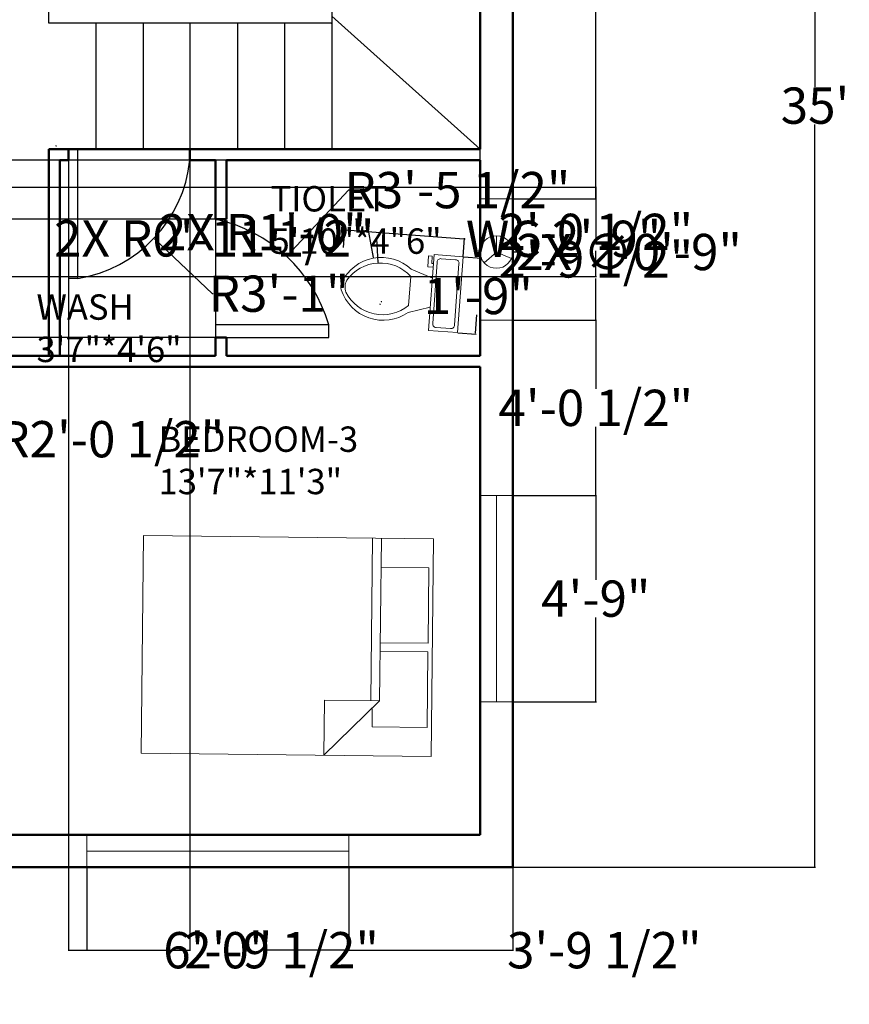
# Model space of a CAD drawing. Units: inches. Extents: x 430 to 924, y 262 to 758.
# Tile 2 of 3: x 695 to 924, y 262 to 534. Entities that reach past the tile are written whole.
import ezdxf

# ---------------------------------------------------------------- set-up
doc = ezdxf.new("R2010")
doc.units = ezdxf.units.IN
doc.header["$MEASUREMENT"] = 0
for name, color, linetype, lineweight in [('A-ANNO-DIMS', 2, 'Continuous', 18), ('A-AREA-IDEN', 7, 'Continuous', 25), ('A-DOOR', 4, 'Continuous', 25), ('A-FLOR-FIXT', 9, 'Continuous', 18), ('A-FLOR-STRS', 7, 'Continuous', 25), ('A-FURN', 9, 'Continuous', 18), ('A-GLAZ', 3, 'Continuous', 18), ('A-WALL', 7, 'Continuous', 50), ('M-HVAC-EQPM', 4, 'Continuous', 18)]:
    doc.layers.add(name, color=color, linetype=linetype, lineweight=lineweight)
doc.styles.get("Standard").update_dxf_attribs({"font": 'arial.ttf'})
doc.dimstyles.get("Standard").update_dxf_attribs({"dimtxt": 10, "dimasz": 0.18, "dimexe": 0.18, "dimexo": 0.0625, "dimgap": 0.09, "dimtad": 0, "dimtih": 1, "dimtoh": 1, "dimdec": 0, "dimzin": 0, "dimdsep": 46, "dimlunit": 3, "dimtxsty": 'Standard', "dimcen": 0.09, "dimadec": 0, "dimazin": 0, "dimtfac": 1, "dimtdec": 0, "dimtofl": 0, "dimtmove": 0, "dimatfit": 3, "dimfxl": 1, "dimtolj": 1, "dimtzin": 0, "dimarcsym": 0})

# ---------------------------------------------------------------- blocks, each defined once
blk = doc.blocks.new('Bed - Queen')
for p, q in [((0, -80.00003), (0, 0)), ((0, 0), (59.99999, 0)), ((59.99999, 0), (59.99999, -80.00003)), ((7.99999, -1.2), (28.79998, -1.2)), ((7.99999, -14.4), (7.99999, -1.2)), ((28.79998, -1.2), (28.79998, -14.4)), ((31.19999, -1.2), (51.99999, -1.2)), ((31.19999, -14.4), (31.19999, -1.2)), ((51.99999, -1.2), (51.99999, -16.4)), ((0, -14.4), (44.8, -14.4)), ((59.99999, -29.6), (44.8, -14.4)), ((44.8, -14.4), (44.8, -29.6)), ((44.8, -16.8), (0, -16.8)), ((51.99999, -16.4), (46.79936, -16.4)), ((44.8, -29.6), (59.99999, -29.6)), ((59.99999, -80.00003), (0, -80.00003))]:
    blk.add_line(p, q)
blk = doc.blocks.new('Toilet - top')
for p, q in [((9.5, -6), (9.5, -2)), ((-8, -8.5), (-8, -8)), ((-7, -8), (-7, -9.5)), ((-4, -8), (-6, -14)), ((4, -8), (6, -14)), ((-10, -8.5), (-8, -8.5)), ((-10, -9.5), (-10, -8.5)), ((-7, -9.5), (-10, -9.5)), ((4, -14), (-4, -14))]:
    blk.add_line(p, q)
blk.add_lwpolyline([(10.5, -8), (10.5, 0), (-10.5, 0), (-10.5, -8)], close=True)
for points in [[(-9.5, -2), (-9.5, -6)], [(8.5, -1), (-8.5, -1)], [(-8.5, -7), (8.5, -7)]]:
    blk.add_lwpolyline(points)
for centre, radius, start, end in [((-8.62, -1.88), 0.884, 81.8699, 188.1301), ((8.62, -1.88), 0.884, 351.8699, 98.1301), ((-8.62, -6.12), 0.884, 171.8699, 278.1301), ((8.62, -6.12), 0.884, 261.8699, 8.1301), ((3.52, -21.58), 12.17, 141.4691, 247.9714), ((4.2, -21.82), 11.33, 136.3677, 238.9468), ((-3.52, -21.58), 12.17, 292.0284, 38.5307), ((-4.2, -21.82), 11.33, 301.053, 43.6321), ((0, -27.88), 4, 245.7318, 294.2682), ((0, -29), 4, 254.8605, 285.1395)]:
    blk.add_arc(centre, radius, start, end)
blk = doc.blocks.new('*D6')
at = {"layer": 'A-ANNO-DIMS', "color": 0, "lineweight": -2, "transparency": 16777216}
for p, q in [((831.38, 720.05), (914.81, 720.05)), ((914.63, 719.87), (914.63, 515.25)), ((914.63, 300.23), (914.63, 504.86)), ((831.38, 300.05), (914.81, 300.05))]:
    blk.add_line(p, q, dxfattribs=at)
at = {"layer": 'A-ANNO-DIMS', "color": 0, "transparency": 16777216}
for points in [[(914.6, 719.87), (914.66, 719.87), (914.63, 720.05)], [(914.6, 300.23), (914.66, 300.23), (914.63, 300.05)]]:
    blk.add_solid(points, dxfattribs=at)
at = {"layer": 'Defpoints', "color": 0, "transparency": 16777216}
for p in [(831.32, 720.05), (831.32, 300.05), (914.63, 300.05)]:
    blk.add_point(p, dxfattribs=at)
at = {"layer": 'A-ANNO-DIMS', "color": 0, "transparency": 16777216, "insert": (914.63, 510.05), "char_height": 10, "attachment_point": 5}
blk.add_mtext("\\A1;35'", dxfattribs=at)
blk = doc.blocks.new('*D13')
at = {"layer": 'A-ANNO-DIMS', "color": 0, "lineweight": -2, "transparency": 16777216}
for p, q in [((784.63, 470.89), (785, 475.95)), ((785.17, 475.76), (817.77, 473.36)), ((817.59, 468.46), (817.96, 473.52)), ((817.95, 473.34), (818.13, 473.33))]:
    blk.add_line(p, q, dxfattribs=at)
at = {"layer": 'A-ANNO-DIMS', "color": 0, "transparency": 16777216}
for points in [[(785.17, 475.79), (785.17, 475.73), (784.99, 475.77)], [(817.77, 473.39), (817.77, 473.33), (817.95, 473.34)]]:
    blk.add_solid(points, dxfattribs=at)
at = {"layer": 'Defpoints', "color": 0, "transparency": 16777216}
for p in [(817.95, 473.34), (784.63, 470.83), (817.58, 468.4)]:
    blk.add_point(p, dxfattribs=at)
at = {"layer": 'A-ANNO-DIMS', "color": 0, "transparency": 16777216, "insert": (845.29, 473.33), "char_height": 10, "attachment_point": 5}
blk.add_mtext('\\A1;WC 2\'-9"', dxfattribs=at)
blk = doc.blocks.new('*D14')
at = {"layer": 'A-ANNO-DIMS', "color": 0, "lineweight": -2, "transparency": 16777216}
for p, q in [((817.65, 468.39), (822.71, 468.02)), ((822.51, 467.85), (822.14, 462.76)), ((821, 447.27), (821.37, 452.37)), ((816.1, 447.45), (821.16, 447.08))]:
    blk.add_line(p, q, dxfattribs=at)
at = {"layer": 'A-ANNO-DIMS', "color": 0, "transparency": 16777216}
for points in [[(822.48, 467.86), (822.54, 467.85), (822.53, 468.03)], [(820.97, 447.27), (821.03, 447.27), (820.98, 447.09)]]:
    blk.add_solid(points, dxfattribs=at)
at = {"layer": 'Defpoints', "color": 0, "transparency": 16777216}
for p in [(817.58, 468.4), (816.04, 447.46), (820.98, 447.09)]:
    blk.add_point(p, dxfattribs=at)
at = {"layer": 'A-ANNO-DIMS', "color": 0, "transparency": 16777216, "insert": (821.76, 457.56), "char_height": 10, "attachment_point": 5}
blk.add_mtext('\\A1;1\'-9"', dxfattribs=at)
blk = doc.blocks.new('*D21')
at = {"layer": 'A-ANNO-DIMS', "color": 0, "lineweight": -2, "transparency": 16777216}
for p, q in [((831.38, 607.32), (854.35, 607.32)), ((854.17, 607.14), (854.17, 551.05)), ((854.17, 484.56), (854.17, 540.65)), ((831.38, 484.38), (854.35, 484.38))]:
    blk.add_line(p, q, dxfattribs=at)
at = {"layer": 'A-ANNO-DIMS', "color": 0, "transparency": 16777216}
for points in [[(854.14, 607.14), (854.2, 607.14), (854.17, 607.32)], [(854.14, 484.56), (854.2, 484.56), (854.17, 484.38)]]:
    blk.add_solid(points, dxfattribs=at)
at = {"layer": 'Defpoints', "color": 0, "transparency": 16777216}
for p in [(831.32, 607.32), (831.32, 484.38), (854.17, 484.38)]:
    blk.add_point(p, dxfattribs=at)
at = {"layer": 'A-ANNO-DIMS', "color": 0, "transparency": 16777216, "insert": (854.17, 545.85), "char_height": 10, "attachment_point": 5}
blk.add_mtext('\\A1;10\'-3"', dxfattribs=at)
blk = doc.blocks.new('*D22')
at = {"layer": 'A-ANNO-DIMS', "color": 0, "lineweight": -2, "transparency": 16777216}
for p, q in [((831.38, 484.38), (854.35, 484.38)), ((854.17, 484.2), (854.17, 472.9)), ((854.17, 451.07), (854.17, 462.38)), ((831.38, 450.89), (854.35, 450.89))]:
    blk.add_line(p, q, dxfattribs=at)
at = {"layer": 'A-ANNO-DIMS', "color": 0, "transparency": 16777216}
for points in [[(854.14, 484.2), (854.2, 484.2), (854.17, 484.38)], [(854.14, 451.07), (854.2, 451.07), (854.17, 450.89)]]:
    blk.add_solid(points, dxfattribs=at)
at = {"layer": 'Defpoints', "color": 0, "transparency": 16777216}
for p in [(831.32, 484.38), (831.32, 450.89), (854.17, 450.89)]:
    blk.add_point(p, dxfattribs=at)
at = {"layer": 'A-ANNO-DIMS', "color": 0, "transparency": 16777216, "insert": (854.17, 467.64), "char_height": 10, "attachment_point": 5}
blk.add_mtext('\\A1;2\'-9 1/2"', dxfattribs=at)
blk = doc.blocks.new('*D23')
at = {"layer": 'A-ANNO-DIMS', "color": 0, "lineweight": -2, "transparency": 16777216}
for p, q in [((831.38, 450.89), (854.35, 450.89)), ((854.17, 450.71), (854.17, 431.98)), ((854.17, 402.73), (854.17, 421.46)), ((831.38, 402.55), (854.35, 402.55))]:
    blk.add_line(p, q, dxfattribs=at)
at = {"layer": 'A-ANNO-DIMS', "color": 0, "transparency": 16777216}
for points in [[(854.14, 450.71), (854.2, 450.71), (854.17, 450.89)], [(854.14, 402.73), (854.2, 402.73), (854.17, 402.55)]]:
    blk.add_solid(points, dxfattribs=at)
at = {"layer": 'Defpoints', "color": 0, "transparency": 16777216}
for p in [(831.32, 450.89), (831.32, 402.55), (854.17, 402.55)]:
    blk.add_point(p, dxfattribs=at)
at = {"layer": 'A-ANNO-DIMS', "color": 0, "transparency": 16777216, "insert": (854.17, 426.72), "char_height": 10, "attachment_point": 5}
blk.add_mtext('\\A1;4\'-0 1/2"', dxfattribs=at)
blk = doc.blocks.new('*D24')
at = {"layer": 'A-ANNO-DIMS', "color": 0, "lineweight": -2, "transparency": 16777216}
for p, q in [((831.38, 402.55), (854.35, 402.55)), ((854.17, 402.37), (854.17, 379.33)), ((854.17, 345.89), (854.17, 368.93)), ((831.38, 345.71), (854.35, 345.71))]:
    blk.add_line(p, q, dxfattribs=at)
at = {"layer": 'A-ANNO-DIMS', "color": 0, "transparency": 16777216}
for points in [[(854.14, 402.37), (854.2, 402.37), (854.17, 402.55)], [(854.14, 345.89), (854.2, 345.89), (854.17, 345.71)]]:
    blk.add_solid(points, dxfattribs=at)
at = {"layer": 'Defpoints', "color": 0, "transparency": 16777216}
for p in [(831.32, 402.55), (831.32, 345.71), (854.17, 345.71)]:
    blk.add_point(p, dxfattribs=at)
at = {"layer": 'A-ANNO-DIMS', "color": 0, "transparency": 16777216, "insert": (854.17, 374.13), "char_height": 10, "attachment_point": 5}
blk.add_mtext('\\A1;4\'-9"', dxfattribs=at)
blk = doc.blocks.new('*D31')
at = {"layer": 'A-ANNO-DIMS', "color": 0, "lineweight": -2, "transparency": 16777216}
for p, q in [((786.02, 299.99), (786.02, 277.02)), ((831.32, 299.99), (831.32, 277.02)), ((786.2, 277.2), (831.14, 277.2)), ((831.32, 277.2), (831.5, 277.2))]:
    blk.add_line(p, q, dxfattribs=at)
at = {"layer": 'A-ANNO-DIMS', "color": 0, "transparency": 16777216}
for points in [[(786.2, 277.23), (786.2, 277.17), (786.02, 277.2)], [(831.14, 277.23), (831.14, 277.17), (831.32, 277.2)]]:
    blk.add_solid(points, dxfattribs=at)
at = {"layer": 'Defpoints', "color": 0, "transparency": 16777216}
for p in [(786.02, 300.05), (831.32, 300.05), (831.32, 277.2)]:
    blk.add_point(p, dxfattribs=at)
at = {"layer": 'A-ANNO-DIMS', "color": 0, "transparency": 16777216, "insert": (856.52, 277.2), "char_height": 10, "attachment_point": 5}
blk.add_mtext('\\A1;3\'-9 1/2"', dxfattribs=at)
blk = doc.blocks.new('*D32')
at = {"layer": 'A-ANNO-DIMS', "color": 0, "lineweight": -2, "transparency": 16777216}
for p, q in [((713.84, 299.99), (713.84, 277.02)), ((786.02, 299.99), (786.02, 277.02)), ((714.02, 277.2), (736.52, 277.2)), ((785.84, 277.2), (763.34, 277.2))]:
    blk.add_line(p, q, dxfattribs=at)
at = {"layer": 'A-ANNO-DIMS', "color": 0, "transparency": 16777216}
for points in [[(714.02, 277.23), (714.02, 277.17), (713.84, 277.2)], [(785.84, 277.23), (785.84, 277.17), (786.02, 277.2)]]:
    blk.add_solid(points, dxfattribs=at)
at = {"layer": 'Defpoints', "color": 0, "transparency": 16777216}
for p in [(713.84, 300.05), (786.02, 300.05), (786.02, 277.2)]:
    blk.add_point(p, dxfattribs=at)
at = {"layer": 'A-ANNO-DIMS', "color": 0, "transparency": 16777216, "insert": (749.93, 277.2), "char_height": 10, "attachment_point": 5}
blk.add_mtext('\\A1;6\'-0"', dxfattribs=at)
blk = doc.blocks.new('*D39')
at = {"layer": 'A-ANNO-DIMS', "color": 0, "lineweight": -2, "transparency": 16777216}
for p, q in [((752.25, 478.73), (460.24, 478.73)), ((460.42, 478.55), (460.42, 467.71)), ((460.42, 446.34), (460.42, 457.18)), ((752.25, 446.16), (460.24, 446.16))]:
    blk.add_line(p, q, dxfattribs=at)
at = {"layer": 'A-ANNO-DIMS', "color": 0, "transparency": 16777216}
for points in [[(460.39, 478.55), (460.45, 478.55), (460.42, 478.73)], [(460.39, 446.34), (460.45, 446.34), (460.42, 446.16)]]:
    blk.add_solid(points, dxfattribs=at)
at = {"layer": 'Defpoints', "color": 0, "transparency": 16777216}
for p in [(460.42, 478.73), (752.32, 478.73), (752.32, 446.16)]:
    blk.add_point(p, dxfattribs=at)
at = {"layer": 'A-ANNO-DIMS', "color": 0, "transparency": 16777216, "insert": (460.42, 462.44), "char_height": 10, "attachment_point": 5}
blk.add_mtext('\\A1;2\'-8 1/2"', dxfattribs=at)
blk = doc.blocks.new('*D40')
at = {"layer": 'A-ANNO-DIMS', "color": 0, "lineweight": -2, "transparency": 16777216}
for p, q in [((752.25, 495.05), (460.24, 495.05)), ((460.42, 494.87), (460.42, 492.15)), ((460.42, 478.91), (460.42, 481.63)), ((752.25, 478.73), (460.24, 478.73))]:
    blk.add_line(p, q, dxfattribs=at)
at = {"layer": 'A-ANNO-DIMS', "color": 0, "transparency": 16777216}
for points in [[(460.39, 494.87), (460.45, 494.87), (460.42, 495.05)], [(460.39, 478.91), (460.45, 478.91), (460.42, 478.73)]]:
    blk.add_solid(points, dxfattribs=at)
at = {"layer": 'Defpoints', "color": 0, "transparency": 16777216}
for p in [(460.42, 495.05), (752.32, 495.05), (752.32, 478.73)]:
    blk.add_point(p, dxfattribs=at)
at = {"layer": 'A-ANNO-DIMS', "color": 0, "transparency": 16777216, "insert": (460.42, 486.89), "char_height": 10, "attachment_point": 5}
blk.add_mtext('\\A1;1\'-4 1/2"', dxfattribs=at)
blk = doc.blocks.new('*D41')
at = {"layer": 'A-ANNO-DIMS', "color": 0, "lineweight": -2, "transparency": 16777216}
for p, q in [((822.32, 484.44), (822.32, 743.09)), ((822.5, 742.91), (831.14, 742.91)), ((831.32, 484.44), (831.32, 743.09)), ((831.32, 742.91), (831.5, 742.91))]:
    blk.add_line(p, q, dxfattribs=at)
at = {"layer": 'A-ANNO-DIMS', "color": 0, "transparency": 16777216}
for points in [[(822.5, 742.94), (822.5, 742.88), (822.32, 742.91)], [(831.14, 742.94), (831.14, 742.88), (831.32, 742.91)]]:
    blk.add_solid(points, dxfattribs=at)
at = {"layer": 'Defpoints', "color": 0, "transparency": 16777216}
for p in [(831.32, 742.91), (822.32, 484.38), (831.32, 484.38)]:
    blk.add_point(p, dxfattribs=at)
at = {"layer": 'A-ANNO-DIMS', "color": 0, "transparency": 16777216, "insert": (844.88, 742.91), "char_height": 10, "attachment_point": 5}
blk.add_mtext('\\A1;0\'-9"', dxfattribs=at)
blk = doc.blocks.new('*D44')
at = {"layer": 'A-ANNO-DIMS', "color": 0, "lineweight": -2, "transparency": 16777216}
for p, q in [((567.38, 487.53), (854.35, 487.53)), ((854.17, 487.35), (854.17, 480.5)), ((854.17, 463.13), (854.17, 469.98)), ((567.38, 462.95), (854.35, 462.95))]:
    blk.add_line(p, q, dxfattribs=at)
at = {"layer": 'A-ANNO-DIMS', "color": 0, "transparency": 16777216}
for points in [[(854.14, 487.35), (854.2, 487.35), (854.17, 487.53)], [(854.14, 463.13), (854.2, 463.13), (854.17, 462.95)]]:
    blk.add_solid(points, dxfattribs=at)
at = {"layer": 'Defpoints', "color": 0, "transparency": 16777216}
for p in [(567.32, 487.53), (854.17, 487.53), (567.32, 462.95)]:
    blk.add_point(p, dxfattribs=at)
at = {"layer": 'A-ANNO-DIMS', "color": 0, "transparency": 16777216, "insert": (854.17, 475.24), "char_height": 10, "attachment_point": 5}
blk.add_mtext('\\A1;2\'-0 1/2"', dxfattribs=at)
blk = doc.blocks.new('*D51')
at = {"layer": 'A-ANNO-DIMS', "color": 0, "lineweight": -2, "transparency": 16777216}
for p, q in [((708.72, 497.99), (708.72, 277.02)), ((742.24, 497.99), (742.24, 277.02)), ((708.9, 277.2), (742.06, 277.2)), ((742.24, 277.2), (742.42, 277.2))]:
    blk.add_line(p, q, dxfattribs=at)
at = {"layer": 'A-ANNO-DIMS', "color": 0, "transparency": 16777216}
for points in [[(708.9, 277.23), (708.9, 277.17), (708.72, 277.2)], [(742.06, 277.23), (742.06, 277.17), (742.24, 277.2)]]:
    blk.add_solid(points, dxfattribs=at)
at = {"layer": 'Defpoints', "color": 0, "transparency": 16777216}
for p in [(708.72, 498.05), (742.24, 498.05), (742.24, 277.2)]:
    blk.add_point(p, dxfattribs=at)
at = {"layer": 'A-ANNO-DIMS', "color": 0, "transparency": 16777216, "insert": (767.53, 277.2), "char_height": 10, "attachment_point": 5}
blk.add_mtext('\\A1;2\'-9 1/2"', dxfattribs=at)
blk = doc.blocks.new('*D57')
at = {"layer": 'A-ANNO-DIMS', "color": 0, "lineweight": -2, "transparency": 16777216}
for p, q in [((664.61, 447.63), (664.79, 447.63)), ((664.7, 447.54), (664.7, 447.72)), ((690.53, 418.08), (680.96, 429.02)), ((690.71, 418.08), (690.53, 418.08))]:
    blk.add_line(p, q, dxfattribs=at)
at = {"layer": 'A-ANNO-DIMS', "color": 0, "transparency": 16777216}
blk.add_solid([(680.98, 429.04), (680.94, 429), (680.84, 429.16)], dxfattribs=at)
at = {"layer": 'Defpoints', "color": 0, "transparency": 16777216}
for p in [(664.7, 447.63), (680.84, 429.16)]:
    blk.add_point(p, dxfattribs=at)
at = {"layer": 'A-ANNO-DIMS', "color": 0, "transparency": 16777216, "insert": (720.53, 418.08), "char_height": 10, "attachment_point": 5}
blk.add_mtext('\\A1;R2\'-0 1/2"', dxfattribs=at)
blk = doc.blocks.new('*D58')
at = {"layer": 'A-ANNO-DIMS', "color": 0, "lineweight": -2, "transparency": 16777216}
for p, q in [((705.3, 498.94), (705.48, 498.94)), ((705.39, 498.85), (705.39, 499.03)), ((748.45, 458.2), (732.43, 473.35)), ((748.63, 458.2), (748.45, 458.2))]:
    blk.add_line(p, q, dxfattribs=at)
at = {"layer": 'A-ANNO-DIMS', "color": 0, "transparency": 16777216}
blk.add_solid([(732.45, 473.37), (732.41, 473.33), (732.3, 473.47)], dxfattribs=at)
at = {"layer": 'Defpoints', "color": 0, "transparency": 16777216}
for p in [(705.39, 498.94), (732.3, 473.47)]:
    blk.add_point(p, dxfattribs=at)
at = {"layer": 'A-ANNO-DIMS', "color": 0, "transparency": 16777216, "insert": (766.8, 458.2), "char_height": 10, "attachment_point": 5}
blk.add_mtext('\\A1;R3\'-1"', dxfattribs=at)
blk = doc.blocks.new('*D59')
at = {"layer": 'A-ANNO-DIMS', "color": 0, "lineweight": -2, "transparency": 16777216}
for p, q in [((785.99, 486.76), (769.05, 468.6)), ((786.17, 486.76), (785.99, 486.76)), ((740.39, 437.98), (740.57, 437.98)), ((740.48, 437.89), (740.48, 438.07))]:
    blk.add_line(p, q, dxfattribs=at)
at = {"layer": 'A-ANNO-DIMS', "color": 0, "transparency": 16777216}
blk.add_solid([(769.03, 468.62), (769.07, 468.58), (768.93, 468.46)], dxfattribs=at)
at = {"layer": 'Defpoints', "color": 0, "transparency": 16777216}
for p in [(768.93, 468.46), (740.48, 437.98)]:
    blk.add_point(p, dxfattribs=at)
at = {"layer": 'A-ANNO-DIMS', "color": 0, "transparency": 16777216, "insert": (815.99, 486.76), "char_height": 10, "attachment_point": 5}
blk.add_mtext('\\A1;R3\'-5 1/2"', dxfattribs=at)
blk = doc.blocks.new('*D60')
at = {"layer": 'A-ANNO-DIMS', "color": 0, "lineweight": -2, "transparency": 16777216}
for p, q in [((791.3, 475.15), (791.48, 475.15)), ((791.48, 475.15), (792.78, 468.15)), ((795.03, 455.91), (795.03, 456.09)), ((794.94, 456), (795.12, 456))]:
    blk.add_line(p, q, dxfattribs=at)
at = {"layer": 'A-ANNO-DIMS', "color": 0, "transparency": 16777216}
blk.add_solid([(792.81, 468.15), (792.75, 468.14), (792.81, 467.97)], dxfattribs=at)
at = {"layer": 'Defpoints', "color": 0, "transparency": 16777216}
for p in [(792.81, 467.97), (795.03, 456)]:
    blk.add_point(p, dxfattribs=at)
at = {"layer": 'A-ANNO-DIMS', "color": 0, "transparency": 16777216, "insert": (762.31, 475.15), "char_height": 10, "attachment_point": 5}
blk.add_mtext('\\A1;2X R1\'-0"', dxfattribs=at)
blk = doc.blocks.new('*D61')
at = {"layer": 'A-ANNO-DIMS', "color": 0, "lineweight": -2, "transparency": 16777216}
for p, q in [((793.48, 473.44), (793.66, 473.44)), ((793.66, 473.44), (794.05, 466.83)), ((794.66, 455.34), (794.84, 455.34)), ((794.75, 455.25), (794.75, 455.43))]:
    blk.add_line(p, q, dxfattribs=at)
at = {"layer": 'A-ANNO-DIMS', "color": 0, "transparency": 16777216}
blk.add_solid([(794.08, 466.83), (794.02, 466.83), (794.07, 466.65)], dxfattribs=at)
at = {"layer": 'Defpoints', "color": 0, "transparency": 16777216}
for p in [(794.07, 466.65), (794.75, 455.34)]:
    blk.add_point(p, dxfattribs=at)
at = {"layer": 'A-ANNO-DIMS', "color": 0, "transparency": 16777216, "insert": (748.95, 473.44), "char_height": 10, "attachment_point": 5}
blk.add_mtext('\\A1;2X R0\'-11 1/2"', dxfattribs=at)
blk = doc.blocks.new('*D62')
at = {"layer": 'A-ANNO-DIMS', "color": 0, "lineweight": -2, "transparency": 16777216}
for p, q in [((826.68, 469.69), (826.86, 469.69)), ((826.77, 469.6), (826.77, 469.78)), ((833.97, 469.69), (831.45, 469.69))]:
    blk.add_line(p, q, dxfattribs=at)
at = {"layer": 'A-ANNO-DIMS', "color": 0, "transparency": 16777216}
blk.add_solid([(831.45, 469.72), (831.45, 469.66), (831.27, 469.69)], dxfattribs=at)
at = {"layer": 'Defpoints', "color": 0, "transparency": 16777216}
for p in [(822.27, 469.69), (831.27, 469.69)]:
    blk.add_point(p, dxfattribs=at)
at = {"layer": 'A-ANNO-DIMS', "color": 0, "transparency": 16777216, "insert": (863.36, 469.69), "char_height": 10, "attachment_point": 5}
blk.add_mtext('\\A1;2X ∅0\'-9"', dxfattribs=at)

msp = doc.modelspace()

# ---------------------------------------------------------------- linework, layer by layer
at = {"layer": 'A-DOOR'}
for p, q in [((711.31, 462.36), (711.31, 498.05)), ((708.72, 495.05), (708.72, 462.36)), ((749.32, 478.73), (749.32, 446.16)), ((711.31, 462.36), (708.72, 462.36)), ((780.52, 449.61), (749.32, 449.61)), ((780.52, 446.16), (780.52, 449.61)), ((752.32, 446.16), (780.52, 446.16))]:
    msp.add_line(p, q, dxfattribs=at)
for centre, radius, start, end in [((705.39, 498.94), 37.05, 279.1888, 353.9847), ((740.48, 437.98), 41.7, 16.2075, 77.7707)]:
    msp.add_arc(centre, radius, start, end, dxfattribs=at)
at = {"layer": 'A-FLOR-STRS'}
for p, q in [((703.32, 532.81), (703.32, 537.05)), ((781.35, 537.05), (781.35, 498.05)), ((781.16, 532.81), (703.32, 532.81)), ((716.32, 532.81), (716.32, 498.05)), ((729.35, 532.81), (729.35, 498.05)), ((742.24, 532.81), (742.24, 498.05)), ((755.35, 532.81), (755.35, 498.05)), ((768.35, 532.81), (768.35, 498.05)), ((781.16, 532.81), (781.35, 532.81)), ((781.35, 534.67), (822.32, 498.05))]:
    msp.add_line(p, q, dxfattribs=at)
at = {"layer": 'A-GLAZ'}
for p, q in [((822.32, 484.38), (831.32, 484.38)), ((822.32, 450.89), (831.32, 450.89)), ((822.32, 402.55), (831.32, 402.55)), ((826.82, 402.55), (826.82, 345.71)), ((822.32, 345.71), (831.32, 345.71)), ((713.84, 309.05), (713.84, 300.05)), ((786.02, 309.05), (786.02, 300.05)), ((713.84, 304.55), (786.02, 304.55))]:
    msp.add_line(p, q, dxfattribs=at)
at = {"layer": 'A-WALL'}
for p, q in [((822.32, 576.05), (822.32, 498.05)), ((706.32, 498.05), (703.32, 498.05)), ((703.32, 498.05), (703.32, 495.05)), ((706.32, 498.05), (822.32, 498.05)), ((708.72, 495.05), (708.72, 498.05)), ((742.24, 498.05), (742.24, 495.05)), ((703.32, 495.05), (703.32, 441.05)), ((706.32, 495.05), (708.72, 495.05)), ((706.32, 495.05), (706.32, 441.05)), ((742.24, 495.05), (749.32, 495.05)), ((749.32, 495.05), (749.32, 478.73)), ((752.32, 495.05), (752.32, 478.73)), ((752.32, 495.05), (822.32, 495.05)), ((822.32, 495.05), (822.32, 441.05)), ((749.32, 478.73), (752.32, 478.73)), ((749.32, 446.16), (752.32, 446.16)), ((749.32, 446.16), (749.32, 441.05)), ((752.32, 446.16), (752.32, 441.05)), ((706.32, 441.05), (688.33, 441.05)), ((706.32, 441.05), (749.32, 441.05)), ((752.32, 441.05), (822.32, 441.05)), ((703.32, 438.05), (688.33, 438.05)), ((706.32, 438.05), (703.32, 438.05)), ((706.32, 438.05), (822.32, 438.05)), ((822.32, 438.05), (822.32, 309.05)), ((822.32, 309.05), (664.32, 309.05))]:
    msp.add_line(p, q, dxfattribs=at)
msp.add_lwpolyline([(831.32, 720.05), (831.32, 300.05), (483.32, 300.05), (483.32, 720.05)], close=True, dxfattribs=at)
at = {"layer": 'M-HVAC-EQPM'}
for q in [(826.77, 474.19), (823.4, 466.71), (830.91, 467.91)]:
    msp.add_line((826.77, 469.69), q, dxfattribs=at)
msp.add_circle((826.77, 469.69), 4.5, dxfattribs=at)

# ---------------------------------------------------------------- block references
at = {"layer": 'A-FLOR-FIXT', "rotation": 265.7845713599945}
msp.add_blockref('Toilet - top', (816.81, 457.93), dxfattribs=at)
at = {"layer": 'A-FURN', "rotation": 269.3765262752653}
msp.add_blockref('Bed - Queen', (809.43, 390.63), dxfattribs=at)

# ---------------------------------------------------------------- texts
at = {"layer": 'A-AREA-IDEN', "char_height": 7, "attachment_point": 1}
for s, insert in [('TIOLET\\P5\'10"*4"6"', (764.46, 487.86)), ('WASH\\P3\'7"*4\'6"', (699.92, 458.01)), ('BEDROOM-3\\P13\'7"*11\'3"', (733.57, 421.59))]:
    msp.add_mtext_dynamic_manual_height_columns(s, width=58.4467, gutter_width=1, heights=[0], dxfattribs=dict(at, insert=insert))

# ---------------------------------------------------------------- dimensions: what is measured, and where the dimension line sits
at = {"layer": 'A-ANNO-DIMS'}
for base, p1, p2, picture, middle in [((831.32, 742.91), (822.32, 484.38), (831.32, 484.38), '*D41', (844.88, 742.91)), ((742.24, 277.2), (708.72, 498.05), (742.24, 498.05), '*D51', (767.53, 277.2)), ((786.02, 277.2), (713.84, 300.05), (786.02, 300.05), '*D32', (749.93, 277.2)), ((831.32, 277.2), (786.02, 300.05), (831.32, 300.05), '*D31', (856.52, 277.2))]:
    dim = msp.add_linear_dim(base=base, p1=p1, p2=p2, dimstyle='Standard', override={"dimdec": 1, "dimlfac": 1, "dimrnd": 0, "dimzin": 1, "dimdsep": 46, "dimlunit": 4, "dimfrac": 2}, dxfattribs=at)
    dim.commit()
    dim.dimension.update_dxf_attribs({"geometry": picture, "text_midpoint": middle})
for base, p1, p2, angle, override, picture, middle in [((914.63, 300.05), (831.32, 720.05), (831.32, 300.05), 90, {"dimclrd": 0, "dimclre": 0, "dimclrt": 0}, '*D6', (914.63, 510.05)), ((854.17, 484.38), (831.32, 607.32), (831.32, 484.38), 90, {"dimdec": 1, "dimlfac": 1, "dimrnd": 0, "dimzin": 1, "dimdsep": 46, "dimlunit": 4, "dimfrac": 2}, '*D21', (854.17, 545.85)), ((460.42, 495.05), (752.32, 478.73), (752.32, 495.05), 90, {"dimdec": 1, "dimlfac": 1, "dimrnd": 0, "dimzin": 1, "dimdsep": 46, "dimlunit": 4, "dimfrac": 2}, '*D40', (460.42, 486.89)), ((854.17, 487.53), (567.32, 462.95), (567.32, 487.53), 90, {"dimdec": 1, "dimlfac": 1, "dimrnd": 0, "dimzin": 1, "dimdsep": 46, "dimlunit": 4, "dimfrac": 2}, '*D44', (854.17, 475.24)), ((854.17, 450.89), (831.32, 484.38), (831.32, 450.89), 90, {"dimdec": 1, "dimlfac": 1, "dimrnd": 0, "dimzin": 1, "dimdsep": 46, "dimlunit": 4, "dimfrac": 2}, '*D22', (854.17, 467.64)), ((460.42, 478.73), (752.32, 446.16), (752.32, 478.73), 90, {"dimdec": 1, "dimlfac": 1, "dimrnd": 0, "dimzin": 1, "dimdsep": 46, "dimlunit": 4, "dimfrac": 2}, '*D39', (460.42, 462.44)), ((820.98, 447.09), (817.58, 468.4), (816.04, 447.46), 265.7846, {"dimdec": 1, "dimlfac": 1, "dimrnd": 0, "dimzin": 1, "dimdsep": 46, "dimlunit": 4, "dimfrac": 2}, '*D14', (821.76, 457.56)), ((854.17, 402.55), (831.32, 450.89), (831.32, 402.55), 90, {"dimdec": 1, "dimlfac": 1, "dimrnd": 0, "dimzin": 1, "dimdsep": 46, "dimlunit": 4, "dimfrac": 2}, '*D23', (854.17, 426.72)), ((854.17, 345.71), (831.32, 402.55), (831.32, 345.71), 90, {"dimdec": 1, "dimlfac": 1, "dimrnd": 0, "dimzin": 1, "dimdsep": 46, "dimlunit": 4, "dimfrac": 2}, '*D24', (854.17, 374.13))]:
    dim = msp.add_linear_dim(base=base, p1=p1, p2=p2, angle=angle, dimstyle='Standard', override=override, dxfattribs=at)
    dim.commit()
    dim.dimension.update_dxf_attribs({"geometry": picture, "text_midpoint": middle})
for center, mpoint, picture, middle in [((740.48, 437.98), (768.93, 468.46), '*D59', (815.99, 486.76)), ((705.39, 498.94), (732.3, 473.47), '*D58', (766.8, 458.2)), ((664.7, 447.63), (680.84, 429.16), '*D57', (720.53, 418.08))]:
    dim = msp.add_radius_dim(center=center, mpoint=mpoint, dimstyle='Standard', override={"dimdec": 1, "dimlfac": 1, "dimrnd": 0, "dimzin": 1, "dimdsep": 46, "dimlunit": 4, "dimfrac": 2}, dxfattribs=at)
    dim.commit()
    dim.dimension.update_dxf_attribs({"geometry": picture, "text_midpoint": middle, "dimtype": 164})
for center, mpoint, picture, middle in [((794.75, 455.34), (794.07, 466.65), '*D61', (748.95, 473.44)), ((795.03, 456), (792.81, 467.97), '*D60', (762.31, 475.15))]:
    dim = msp.add_radius_dim(center=center, mpoint=mpoint, text='2X <>', dimstyle='Standard', override={"dimdec": 1, "dimlfac": 1, "dimrnd": 0, "dimzin": 1, "dimdsep": 46, "dimlunit": 4, "dimfrac": 2}, dxfattribs=at)
    dim.commit()
    dim.dimension.update_dxf_attribs({"geometry": picture, "text_midpoint": middle, "dimtype": 164})
dim = msp.add_linear_dim(base=(817.95, 473.34), p1=(784.63, 470.83), p2=(817.58, 468.4), angle=355.7846, text='WC <>', dimstyle='Standard', override={"dimdec": 1, "dimlfac": 1, "dimrnd": 0, "dimzin": 1, "dimdsep": 46, "dimlunit": 4, "dimfrac": 2}, dxfattribs=at)
dim.commit()
dim.dimension.update_dxf_attribs({"geometry": '*D13', "text_midpoint": (845.29, 473.33)})
dim = msp.add_diameter_dim_2p(p1=(822.27, 469.69), p2=(831.27, 469.69), text='2X <>', dimstyle='Standard', override={"dimdec": 1, "dimlfac": 1, "dimrnd": 0, "dimzin": 1, "dimdsep": 46, "dimlunit": 4, "dimfrac": 2}, dxfattribs=at)
dim.commit()
dim.dimension.update_dxf_attribs({"geometry": '*D62', "text_midpoint": (833.97, 469.69), "dimtype": 163})

doc.saveas('drawing.dxf')
